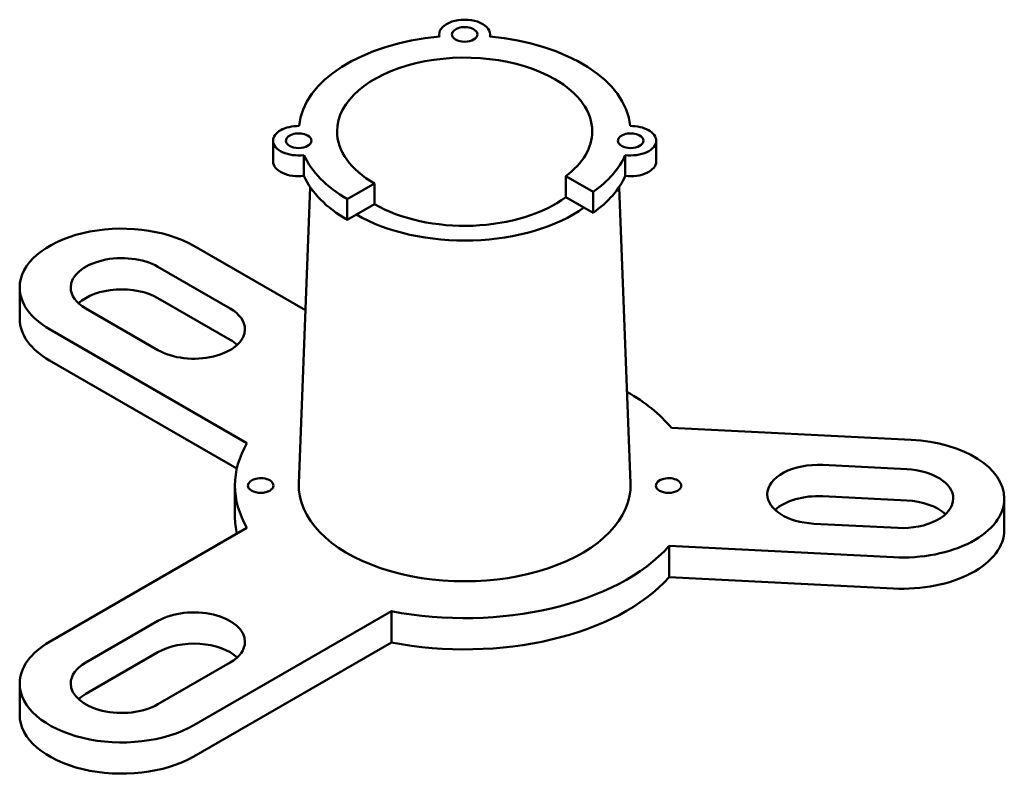
# Model space of a CAD drawing. Units: millimetres. Extents: x 170 to 643, y 16 to 380.
import ezdxf

# ---------------------------------------------------------------- set-up
doc = ezdxf.new("R2010")
doc.units = ezdxf.units.MM
doc.header["$MEASUREMENT"] = 0
doc.layers.add('M-OUTL', color=7, linetype='Continuous', lineweight=50)

msp = doc.modelspace()

# ---------------------------------------------------------------- linework, layer by layer
at = {"layer": 'M-OUTL'}
for p, q in [((371.57, 372.09), (371.57, 373.18)), ((396.06, 372.09), (396.06, 373.18)), ((291.89, 312.18), (291.89, 322.18)), ((475.74, 312.18), (475.74, 322.18)), ((306.7, 305.27), (306.7, 315.27)), ((460.93, 305.27), (460.93, 315.27)), ((445.46, 297.59), (432.38, 305.14)), ((432.38, 295.14), (432.38, 305.14)), ((309.67, 299.94), (304.23, 157.7)), ((327.52, 294.18), (340.52, 301.68)), ((340.52, 291.68), (340.52, 301.68)), ((457.96, 299.94), (463.41, 157.7)), ((327.52, 284.18), (327.52, 294.18)), ((441.1, 290.11), (432.38, 295.14)), ((445.46, 287.59), (445.46, 297.59)), ((331.85, 286.68), (340.52, 291.68)), ((445.46, 287.59), (441.1, 290.11)), ((327.52, 284.18), (331.85, 286.68)), ((307.41, 240.79), (253.91, 271.68)), ((236.59, 261.68), (271.23, 241.68)), ((170.28, 236.68), (170.28, 251.68)), ((236.59, 246.68), (271.23, 226.68)), ((236.59, 221.68), (201.95, 241.68)), ((279.35, 176.99), (184.63, 231.68)), ((274.49, 164.8), (184.63, 216.68)), ((483.02, 184.42), (598.1, 178.61)), ((555.7, 166.55), (595.96, 164.52)), ((273.59, 141.68), (273.59, 156.68)), ((555.7, 151.55), (595.96, 149.52)), ((642.82, 150.43), (642.82, 135.43)), ((591.69, 136.34), (551.43, 138.38)), ((184.63, 81.68), (279.35, 136.37)), ((589.56, 122.25), (481.94, 127.69)), ((481.94, 112.69), (481.94, 127.69)), ((592.61, 122.25), (592.61, 122.25)), ((589.56, 107.25), (481.94, 112.69)), ((592.6, 107.25), (592.6, 107.25)), ((253.91, 41.68), (348.64, 96.37)), ((348.64, 81.37), (348.64, 96.37)), ((236.59, 91.68), (201.95, 71.68)), ((253.91, 26.68), (348.64, 81.37)), ((236.59, 76.68), (201.95, 56.68)), ((236.59, 51.68), (271.23, 71.68)), ((170.28, 46.68), (170.28, 61.68))]:
    msp.add_line(p, q, dxfattribs=at)
for centre, major_axis, start_param, end_param in [((383.82, 373.18), (12.25, 0), 0, 3.141593), ((383.82, 373.18), (6.12, 0), 0.785398, 3.141593), ((383.82, 373.18), (6.12, 0), 0, 0.785398), ((383.82, 326.68), (-79.61, 0), 4.865047, 6.227236), ((383.82, 373.18), (12.25, 0), 3.141593, 3.293866), ((383.82, 373.18), (6.12, 0), 3.141593, 6.283185), ((383.82, 373.18), (12.25, 0), 6.130912, 6.283185), ((383.82, 326.68), (-79.61, 0), 3.197542, 4.559731), ((383.82, 326.68), (61.24, 0), 0.785398, 3.141593), ((383.82, 326.68), (61.24, 0), 0, 0.785398), ((304.14, 322.18), (12.25, 0), 1.555242, 3.141593), ((383.82, 326.68), (61.24, 0), 3.141593, 3.926991), ((383.82, 326.68), (61.24, 0), 5.628156, 6.283185), ((463.49, 322.18), (12.25, 0), 0, 1.58635), ((304.14, 322.18), (12.25, 0), 3.141593, 4.922975), ((304.14, 322.18), (6.12, 0), 0.785398, 3.141593), ((304.14, 322.18), (6.12, 0), 3.141593, 6.283185), ((304.14, 322.18), (6.12, 0), 0, 0.785398), ((463.49, 322.18), (6.12, 0), 0.785398, 3.141593), ((463.49, 322.18), (6.12, 0), 3.141593, 6.283185), ((463.49, 322.18), (12.25, 0), 4.501803, 6.283185), ((463.49, 322.18), (6.12, 0), 0, 0.785398), ((304.14, 312.18), (12.25, 0), 3.141593, 4.922975), ((383.82, 326.68), (-79.61, 0), 0.250981, 0.785398), ((383.82, 326.68), (-79.61, 0), 2.456362, 2.890611), ((463.49, 312.18), (12.25, 0), 4.501803, 6.283185), ((383.82, 316.68), (79.61, 0), 3.392574, 3.926991), ((383.82, 316.68), (79.61, 0), 5.597955, 6.032204), ((383.82, 316.68), (61.24, 0), 3.926991, 5.628156), ((383.82, 316.68), (73.48, 0), 3.926991, 5.606334), ((219.27, 251.68), (48.99, 0), 0.785398, 3.141593), ((219.27, 251.68), (-24.49, 0), 3.926991, 6.283185), ((219.27, 251.68), (48.99, 0), 3.141593, 3.926991), ((219.27, 251.68), (-24.49, 0), 0, 0.785398), ((219.27, 236.68), (-24.49, 0), 3.926991, 5.724195), ((253.91, 231.68), (-24.49, 0), 3.141593, 3.926991), ((219.27, 236.68), (48.99, 0), 3.141593, 3.926991), ((253.91, 231.68), (-24.49, 0), 0.785398, 3.141593), ((253.91, 216.68), (-24.49, 0), 3.700583, 3.926991), ((383.82, 156.68), (-110.23, 0), 3.592607, 3.927478), ((383.82, 156.68), (-110.23, 0), 5.958341, 6.283185), ((593.83, 150.43), (-48.99, 0), 3.141593, 4.625127), ((553.56, 152.46), (-24.49, 0), 4.625127, 6.283185), ((593.83, 150.43), (-24.49, 0), 3.141593, 4.625127), ((383.82, 156.68), (-110.23, 0), 0, 0.324844), ((285.96, 156.68), (6.12, 0), 0.785398, 3.141593), ((285.96, 156.68), (6.12, 0), 3.141593, 6.283185), ((285.96, 156.68), (6.12, 0), 0, 0.785398), ((383.82, 156.68), (79.61, 0), 3.119494, 6.305284), ((481.68, 156.68), (6.12, 0), 0.785398, 3.141593), ((481.68, 156.68), (6.12, 0), 3.141593, 6.283185), ((481.68, 156.68), (6.12, 0), 0, 0.785398), ((553.56, 152.46), (-24.49, 0), 0, 1.483535), ((553.56, 137.46), (-24.49, 0), 4.625127, 5.724194), ((593.83, 150.43), (-48.99, 0), 1.483535, 3.141593), ((593.83, 150.43), (-24.49, 0), 1.483535, 3.141593), ((593.83, 135.43), (-24.49, 0), 3.700584, 4.625127), ((383.82, 141.68), (110.23, 0), 3.141593, 3.269527), ((593.83, 135.43), (-48.99, 0), 1.483535, 3.141593), ((383.82, 156.68), (-110.23, 0), 1.245952, 2.668606), ((383.82, 141.68), (110.23, 0), 4.387545, 5.810199), ((253.91, 81.68), (24.49, 0), 0, 2.356194), ((219.27, 61.68), (48.99, 0), 2.356194, 3.141593), ((253.91, 66.68), (24.49, 0), 0.55899, 2.356194), ((253.91, 81.68), (24.49, 0), 5.497787, 6.283185), ((219.27, 61.68), (24.49, 0), 2.356194, 3.141593), ((219.27, 61.68), (48.99, 0), 3.141593, 5.497787), ((219.27, 61.68), (24.49, 0), 3.141593, 5.497787), ((219.27, 46.68), (24.49, 0), 2.356194, 2.582603), ((219.27, 46.68), (48.99, 0), 3.141593, 5.497787)]:
    msp.add_ellipse(centre, major_axis=major_axis, ratio=0.57735, start_param=start_param, end_param=end_param, dxfattribs=at)

doc.saveas('drawing.dxf')
